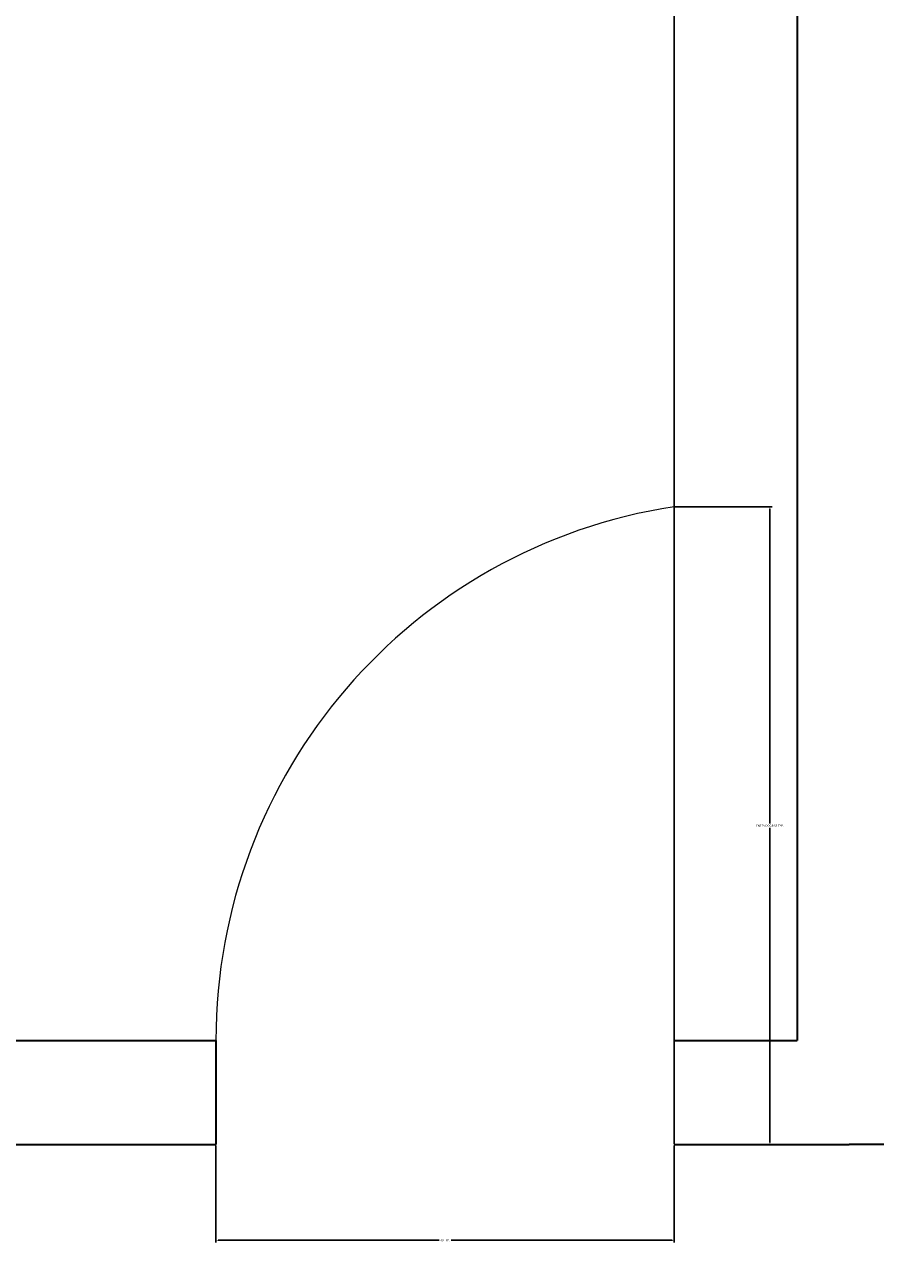
# Model space of a CAD drawing. Units: feet. Extents: x 5816 to 6644, y 25475 to 26788.
# Tile 8 of 23: x 6159 to 6232, y 26158 to 26265. Entities that reach past the tile are written whole.
import ezdxf

# ---------------------------------------------------------------- set-up
doc = ezdxf.new("R2010")
doc.units = ezdxf.units.FT
for name, color, linetype, lineweight in [('A-ANNO-DIMS', 2, 'Continuous', 13), ('A-DOOR', 3, 'Continuous', 18), ('A-WALL', 7, 'Continuous', 35)]:
    doc.layers.add(name, color=color, linetype=linetype, lineweight=lineweight)
doc.styles.get("Standard").update_dxf_attribs({"font": 'arial.ttf'})
doc.dimstyles.get("Standard").update_dxf_attribs({"dimtxt": 0.18, "dimasz": 0.18, "dimexe": 0.18, "dimexo": 0.0625, "dimgap": 0.09, "dimtad": 0, "dimtih": 1, "dimtoh": 1, "dimdec": 4, "dimzin": 0, "dimdsep": 46, "dimtxsty": 'Standard', "dimcen": 0.09, "dimadec": 0, "dimazin": 0, "dimtfac": 1, "dimtdec": 4, "dimtofl": 0, "dimtmove": 0, "dimatfit": 3, "dimfxl": 1, "dimtolj": 1, "dimtzin": 0, "dimarcsym": 0})

# ---------------------------------------------------------------- blocks, each defined once
blk = doc.blocks.new('DOOR-FLAT-ENTRY')
blk.add_line((0, 55.13), (0, 0))
blk.add_arc((7.05, 9.01), 46.66, 98.693, 180)
blk = doc.blocks.new('*D31')
at = {"layer": 'A-ANNO-DIMS', "color": 0, "lineweight": -2, "transparency": 16777216}
for p, q in [((6214.75, 26223.72), (6223.14, 26223.72)), ((6222.96, 26223.54), (6222.96, 26196.33)), ((6222.96, 26168.76), (6222.96, 26195.97)), ((6214.75, 26168.58), (6223.14, 26168.58))]:
    blk.add_line(p, q, dxfattribs=at)
at = {"layer": 'A-ANNO-DIMS', "color": 0, "transparency": 16777216}
for points in [[(6222.93, 26223.54), (6222.99, 26223.54), (6222.96, 26223.72)], [(6222.93, 26168.76), (6222.99, 26168.76), (6222.96, 26168.58)]]:
    blk.add_solid(points, dxfattribs=at)
at = {"layer": 'Defpoints', "color": 0, "transparency": 16777216}
for p in [(6214.69, 26223.72), (6222.96, 26223.72), (6214.69, 26168.58)]:
    blk.add_point(p, dxfattribs=at)
at = {"layer": 'A-ANNO-DIMS', "color": 0, "transparency": 16777216, "insert": (6222.96, 26196.15), "char_height": 0.18, "attachment_point": 5}
blk.add_mtext('\\A1;ENTRY DOOR 55 TYP.', dxfattribs=at)
blk = doc.blocks.new('*D32')
at = {"layer": 'A-ANNO-DIMS', "color": 0, "lineweight": -2, "transparency": 16777216}
for p, q in [((6175.08, 26168.52), (6175.08, 26160.14)), ((6214.69, 26168.52), (6214.69, 26160.14)), ((6175.26, 26160.32), (6194.36, 26160.32)), ((6214.51, 26160.32), (6195.42, 26160.32))]:
    blk.add_line(p, q, dxfattribs=at)
at = {"layer": 'A-ANNO-DIMS', "color": 0, "transparency": 16777216}
for points in [[(6175.26, 26160.35), (6175.26, 26160.29), (6175.08, 26160.32)], [(6214.51, 26160.35), (6214.51, 26160.29), (6214.69, 26160.32)]]:
    blk.add_solid(points, dxfattribs=at)
at = {"layer": 'Defpoints', "color": 0, "transparency": 16777216}
for p in [(6175.08, 26168.58), (6214.69, 26168.58), (6214.69, 26160.32)]:
    blk.add_point(p, dxfattribs=at)
at = {"layer": 'A-ANNO-DIMS', "color": 0, "transparency": 16777216, "insert": (6194.89, 26160.32), "char_height": 0.18, "attachment_point": 5}
blk.add_mtext('\\A1;40 TYP.', dxfattribs=at)
blk = doc.blocks.new('*D60')
at = {"layer": 'A-ANNO-DIMS', "color": 0, "lineweight": -2, "transparency": 16777216}
for p, q in [((6106.98, 26094.4), (6106.98, 26787.91)), ((6107.16, 26787.73), (6224.93, 26787.73)), ((6343.5, 26787.73), (6225.72, 26787.73)), ((6343.68, 26094.4), (6343.68, 26787.91))]:
    blk.add_line(p, q, dxfattribs=at)
at = {"layer": 'A-ANNO-DIMS', "color": 0, "transparency": 16777216}
for points in [[(6107.16, 26787.76), (6107.16, 26787.7), (6106.98, 26787.73)], [(6343.5, 26787.76), (6343.5, 26787.7), (6343.68, 26787.73)]]:
    blk.add_solid(points, dxfattribs=at)
at = {"layer": 'Defpoints', "color": 0, "transparency": 16777216}
for p in [(6343.68, 26787.73), (6106.98, 26094.34), (6343.68, 26094.34)]:
    blk.add_point(p, dxfattribs=at)
at = {"layer": 'A-ANNO-DIMS', "color": 0, "transparency": 16777216, "insert": (6225.33, 26787.73), "char_height": 0.18, "attachment_point": 5}
blk.add_mtext('\\A1;236.7', dxfattribs=at)
blk = doc.blocks.new('*D72')
at = {"layer": 'A-ANNO-DIMS', "color": 0, "lineweight": -2, "transparency": 16777216}
for p, q in [((6214.69, 26168.65), (6214.69, 26787.91)), ((6214.87, 26787.73), (6219.56, 26787.73)), ((6225.13, 26787.73), (6220.44, 26787.73)), ((6225.31, 26177.65), (6225.31, 26787.91))]:
    blk.add_line(p, q, dxfattribs=at)
at = {"layer": 'A-ANNO-DIMS', "color": 0, "transparency": 16777216}
for points in [[(6214.87, 26787.76), (6214.87, 26787.7), (6214.69, 26787.73)], [(6225.13, 26787.76), (6225.13, 26787.7), (6225.31, 26787.73)]]:
    blk.add_solid(points, dxfattribs=at)
at = {"layer": 'Defpoints', "color": 0, "transparency": 16777216}
for p in [(6225.31, 26787.73), (6225.31, 26177.58), (6214.69, 26168.58)]:
    blk.add_point(p, dxfattribs=at)
at = {"layer": 'A-ANNO-DIMS', "color": 0, "transparency": 16777216, "insert": (6220, 26787.73), "char_height": 0.18, "attachment_point": 5}
blk.add_mtext('\\A1;10.621', dxfattribs=at)

msp = doc.modelspace()

# ---------------------------------------------------------------- linework, layer by layer
at = {"layer": 'A-WALL'}
for p, q in [((6225.3119, 26391.0846), (6225.3119, 26177.5846)), ((6056.8119, 26177.5846), (6175.0829, 26177.5846)), ((6175.0829, 26177.5916), (6175.0829, 26168.5846)), ((6214.6905, 26177.5846), (6225.3119, 26177.5846)), ((5962.9781, 26168.5846), (6175.0829, 26168.5846)), ((6214.6905, 26168.5846), (6229.8119, 26168.5846)), ((6244.9332, 26168.5846), (6229.8119, 26168.5846))]:
    msp.add_line(p, q, dxfattribs=at)

# ---------------------------------------------------------------- block references
at = {"layer": 'A-DOOR'}
msp.add_blockref('DOOR-FLAT-ENTRY', (6214.6905, 26168.5846), dxfattribs=at)

# ---------------------------------------------------------------- dimensions: what is measured, and where the dimension line sits
at = {"layer": 'A-ANNO-DIMS'}
for base, p1, p2, override, picture, middle in [((6343.6763, 26787.7346), (6106.9781, 26094.3368), (6343.6763, 26094.3368), {"dimdec": 1, "dimlfac": 1, "dimrnd": 0, "dimzin": 0, "dimdsep": 46, "dimlunit": 2}, '*D60', (6225.3272, 26787.7346)), ((6225.3119, 26787.7346), (6214.6905, 26168.5846), (6225.3119, 26177.5846), {"dimdec": 3, "dimlfac": 1, "dimrnd": 0, "dimzin": 0, "dimdsep": 46, "dimlunit": 2}, '*D72', (6220.0012, 26787.7346))]:
    dim = msp.add_linear_dim(base=base, p1=p1, p2=p2, dimstyle='Standard', override=override, dxfattribs=at)
    dim.commit()
    dim.dimension.update_dxf_attribs({"geometry": picture, "text_midpoint": middle})
dim = msp.add_linear_dim(base=(6222.9602, 26223.7154), p1=(6214.6905, 26168.5846), p2=(6214.6905, 26223.7154), angle=90, text='ENTRY DOOR <> TYP.', dimstyle='Standard', override={"dimdec": 0, "dimlfac": 1, "dimrnd": 0, "dimzin": 0, "dimdsep": 46, "dimlunit": 2}, dxfattribs=at)
dim.commit()
dim.dimension.update_dxf_attribs({"geometry": '*D31', "text_midpoint": (6222.9602, 26196.15)})
dim = msp.add_linear_dim(base=(6214.6905, 26160.315), p1=(6175.0829, 26168.5846), p2=(6214.6905, 26168.5846), text='<> TYP.', dimstyle='Standard', override={"dimdec": 0, "dimlfac": 1, "dimrnd": 0, "dimzin": 0, "dimdsep": 46, "dimlunit": 2}, dxfattribs=at)
dim.commit()
dim.dimension.update_dxf_attribs({"geometry": '*D32', "text_midpoint": (6194.8867, 26160.315)})

doc.saveas('drawing.dxf')
